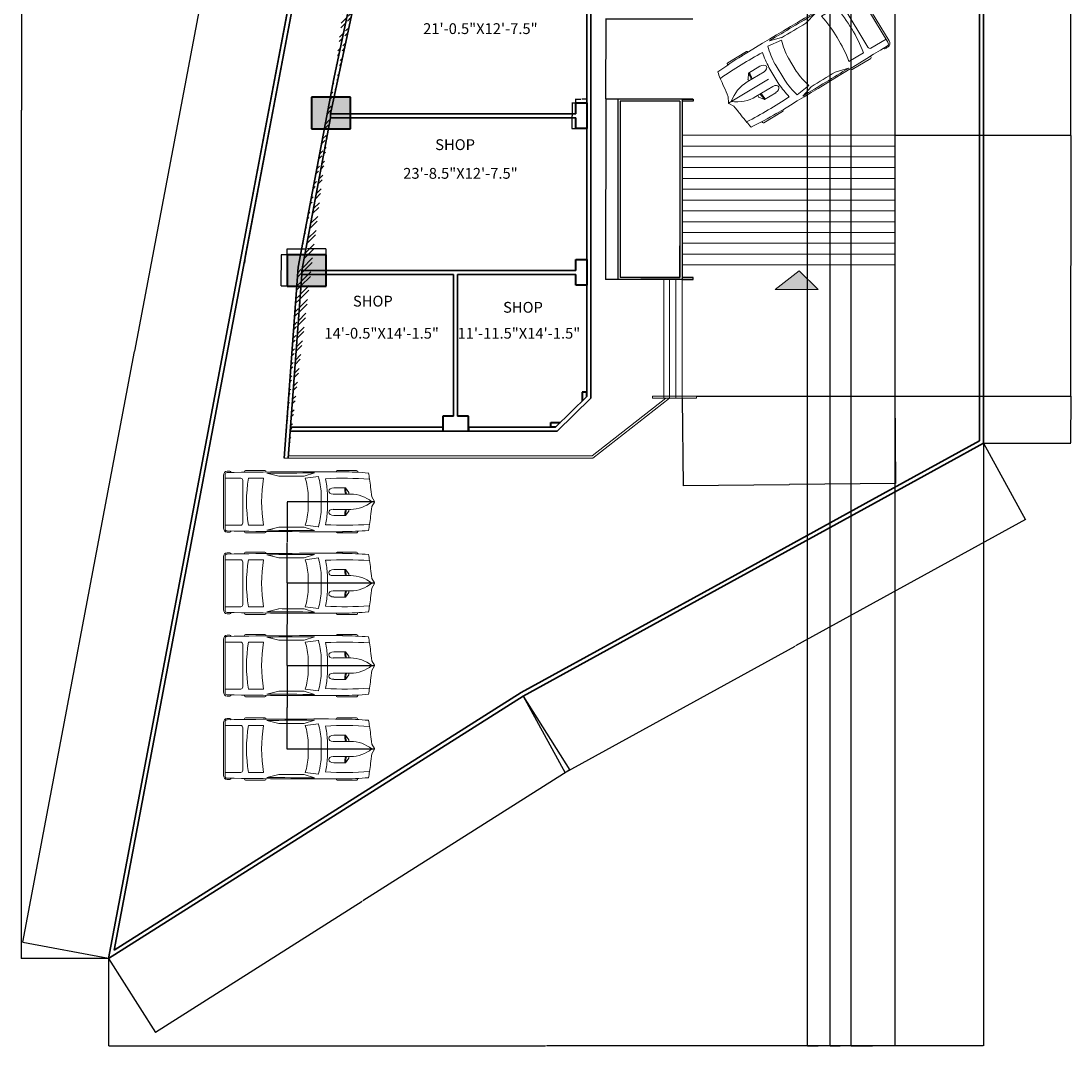
# Model space of a CAD drawing. Units: inches. Extents: x 1563 to 5866, y -225 to 2207.
# Tile 1 of 3: x 2993 to 4159, y -225 to 913. Entities that reach past the tile are written whole.
import ezdxf

# ---------------------------------------------------------------- set-up
doc = ezdxf.new("R2010")
doc.units = ezdxf.units.IN
for name, color, linetype, lineweight in [('A-ANNO-DIMS', 2, 'Continuous', 18), ('A-ANNO-SYMB', 7, 'Continuous', 18), ('A-AREA-IDEN', 7, 'Continuous', 18), ('A-COLS', 1, 'Continuous', 40), ('A-FLOR-STRS', 3, 'Continuous', 18), ('A-WALL', 7, 'Continuous', 35), ('A-WALL-INTR', 7, 'Continuous', 30), ('A-WALL-PATT', 8, 'Continuous', 13), ('C-PKNG', 8, 'Continuous', 25), ('C-PKNG-VEHI', 9, 'Continuous', 13), ('C-PROP', 2, 'Continuous', 35), ('C-SITE-PVMT', 9, 'Continuous', 18)]:
    doc.layers.add(name, color=color, linetype=linetype, lineweight=lineweight)
doc.styles.get("Standard").update_dxf_attribs({"font": 'arial.ttf'})
doc.dimstyles.get("Standard").update_dxf_attribs({"dimtxt": 0.18, "dimasz": 0.18, "dimexe": 0.18, "dimexo": 0.0625, "dimgap": 0.09, "dimtad": 0, "dimtih": 1, "dimtoh": 1, "dimdec": 4, "dimzin": 0, "dimdsep": 46, "dimtxsty": 'Standard', "dimcen": 0.09, "dimadec": 0, "dimazin": 0, "dimtfac": 1, "dimtdec": 4, "dimtofl": 0, "dimtmove": 0, "dimatfit": 3, "dimfxl": 1, "dimtolj": 1, "dimtzin": 0, "dimarcsym": 0})

# ---------------------------------------------------------------- blocks, each defined once
blk = doc.blocks.new('*U2')
for p, q in [((21.1, 37.4), (21.1, 36.8)), ((46.6, 38.9), (22.4, 38.9)), ((47.8, 37.4), (47.8, 37.4)), ((88, 31.9), (74.8, 35.9)), ((134.3, 35.6), (119.3, 31.8)), ((135.5, 37.1), (135.5, 37.4)), ((136.7, 38.9), (160.9, 38.9)), ((162.1, 37.4), (162.1, 36.8)), ((70, 31.5), (86.4, 29.4)), ((138.4, 29.4), (157.2, 29.4)), ((164.5, 26.4), (164.5, -26.4)), ((186.5, 29.4), (167, 29.4)), ((186.5, -33.5), (186.5, 33.5)), ((188.4, -32.8), (188.4, 32.8)), ((32.3, 11.6), (36.1, 17.2)), ((36.1, 17.2), (50.9, 17.2)), ((3.3, 6.1), (0.1, 0.4)), ((29.8, 9.5), (51.7, 9.5)), ((32.1, 9.5), (32.1, 11.2)), ((58.9, -10.8), (58.9, 10.8)), ((66.6, -10.5), (66.6, 10.5)), ((82.7, 8.5), (82.7, -8.5)), ((186.5, -10.5), (186.5, 10.5)), ((0, 0), (51.7, 0)), ((0.1, -0.4), (3.3, -6.1)), ((29.8, -9.5), (51.7, -9.5)), ((32.1, -9.5), (32.1, -11.2)), ((32.3, -11.6), (36.1, -17.2)), ((36.1, -17.2), (50.9, -17.2)), ((86.4, -29.4), (70, -31.5)), ((88, -31.9), (74.8, -35.9)), ((134.3, -35.6), (119.3, -31.8)), ((157.2, -29.4), (138.4, -29.4)), ((167, -29.4), (186.5, -29.4)), ((21.1, -37.4), (21.1, -36.8)), ((46.6, -38.9), (22.4, -38.9)), ((47.8, -37.4), (47.8, -37.4)), ((135.5, -37.1), (135.5, -37.4)), ((136.7, -38.9), (160.9, -38.9)), ((162.1, -37.4), (162.1, -36.8))]:
    blk.add_line(p, q)
for centre, major_axis, ratio, start_param, end_param in [((266, -27.5), (0, 313.3), 0.842304, 1.367076, 1.39176), ((41.2, -490.9), (0, 528.2), 0.842304, 0.00281, 0.075598), ((22.4, 37.4), (0, -1.48), 0.842304, 3.141593, 4.712389), ((64.5, -10555.6), (0, 10593), 0.842304, -0.013397, 0.002797), ((46.6, 37.4), (0, 1.48), 0.842304, -1.570796, 0), ((64.5, -10555.6), (0, -10591.5), 0.842304, 3.133765, 3.140441), ((136.7, 37.4), (0, -1.48), 0.842304, 3.141593, 4.712389), ((160.9, 37.4), (0, 1.48), 0.842304, -1.570796, 0), ((180.6, 35.8), (0, 2.22), 0.842304, -0.013017, 1.249894), ((64.5, -10556.4), (0, 10595.3), 0.842304, -0.013397, -0.013017), ((184, 32.8), (0, -5.25), 0.842304, 1.570796, 3.128196), ((184, 33.5), (0, -2.96), 0.842304, 1.570796, 3.128196), ((259.2, -27.5), (0, -305.3), 0.842304, 4.528606, 4.561838), ((37.5, -594), (0, -623.3), 0.842304, 3.096046, 3.200911), ((134.4, 5.4), (0, -89.8), 0.842304, 4.449482, 4.652344), ((135.3, 5.4), (0, 81.8), 0.842304, 1.245306, 1.50788), ((149.6, 2.8), (0, -79.6), 0.842304, 4.372215, 4.640744), ((95.8, -3666.4), (0, -3698.2), 0.842304, 3.134049, 3.144098), ((17.1, 0), (0, 147), 0.842304, 4.511394, 4.913384), ((35.9, 0), (0, 147), 0.842304, 4.511394, 4.913384), ((167, 26.4), (0, 2.96), 0.842304, 0, 1.570796), ((-204.5, 52.4), (0, -251), 0.842304, 1.385369, 1.434372), ((13, 17), (0, 27.4), 0.842304, 4.435146, 4.718221), ((14.2, 17), (0, 27.4), 0.842304, 4.435146, 4.718221), ((50.8, 13.3), (6.34, -0.36), 0.603834, -1.395552, 1.581315), ((0.6, 0), (0, -0.74), 0.842304, 4.131459, 5.293319), ((29.8, -46.7), (0, 56.2), 0.842304, 0, 0.590319), ((32.7, 11.2), (0, 0.74), 0.842304, 0.879714, 1.570796), ((-204.5, -52.4), (0, 251), 0.842304, -1.434372, -1.385369), ((29.8, 46.7), (0, 56.2), 0.842304, 2.551274, 3.141593), ((32.7, -11.2), (0, -0.74), 0.842304, 4.712389, 5.403472), ((13, -17), (0, -27.4), 0.842304, 1.564964, 1.848039), ((14.2, -17), (0, -27.4), 0.842304, 1.564964, 1.848039), ((134.4, -5.4), (0, -89.8), 0.842304, -1.510751, -1.307889), ((135.3, -5.4), (0, -81.8), 0.842304, -1.50788, -1.245306), ((149.6, -2.8), (0, -79.6), 0.842304, -1.499151, -1.230623), ((259.2, 27.5), (0, 305.3), 0.842304, 1.721348, 1.754579), ((266, 27.5), (0, 313.3), 0.842304, 1.749832, 1.774517), ((37.5, 594), (0, -623.3), 0.842304, -0.059319, 0.045547), ((95.8, 3666.4), (0, -3698.2), 0.842304, -0.002505, 0.007544), ((167, -26.4), (0, -2.96), 0.842304, 4.712389, 6.283185), ((184, -32.8), (0, -5.25), 0.842304, 0.013397, 1.570796), ((184, -33.5), (0, 2.96), 0.842304, 3.15499, 4.712389), ((41.2, 490.9), (0, -528.2), 0.842304, -0.075598, -0.00281), ((22.4, -37.4), (0, 1.48), 0.842304, 1.570796, 3.141593), ((64.5, 10555.6), (0, 10593), 0.842304, 3.138796, 3.15499), ((46.6, -37.4), (0, -1.48), 0.842304, 0, 1.570796), ((64.5, 10555.6), (0, -10591.5), 0.842304, 0.001152, 0.007828), ((136.7, -37.4), (0, -1.48), 0.842304, -1.570796, 0), ((160.9, -37.4), (0, 1.48), 0.842304, 3.141593, 4.712389), ((180.6, -35.8), (0, -2.22), 0.842304, -1.249894, 0.013017), ((64.5, 10556.4), (0, 10595.3), 0.842304, 3.15461, 3.15499)]:
    blk.add_ellipse(centre, major_axis=major_axis, ratio=ratio, start_param=start_param, end_param=end_param)
at = {"extrusion": (0, 0, -1)}
blk.add_ellipse((50.8, -13.3), major_axis=(6.34, 0.36), ratio=0.603834, start_param=-1.395552, end_param=1.581315, dxfattribs=at)
blk = doc.blocks.new('COL-RECT-FILLED')
h = blk.add_hatch(color=256)
h.dxf.hatch_style = 1
h.paths.add_polyline_path([(0, 34.9), (0, 0), (43.4, 0), (43.4, 34.9)])
for p, q in [((43.4, 34.9), (0, 34.9)), ((0, 34.9), (0, 0)), ((43.4, 0), (43.4, 34.9)), ((0, 0), (43.4, 0))]:
    blk.add_line(p, q)
blk = doc.blocks.new('PIER-SHOP-RETURN-2')
for p, q in [((0, 16.5), (0, 28.5)), ((0, 28.5), (12, 28.5)), ((12, 28.5), (12, 12)), ((0, 0), (0, 12)), ((12, 12), (12, 0)), ((12, 0), (0, 0))]:
    blk.add_line(p, q)
blk = doc.blocks.new('*D10')
at = {"layer": 'A-ANNO-DIMS', "color": 0, "lineweight": -2, "transparency": 16777216}
for p, q in [((3288.6, 653.6), (3288.6, 660.2)), ((3288.8, 660), (3309.2, 660)), ((3331.8, 660), (3311.4, 660)), ((3332, 653.6), (3332, 660.2))]:
    blk.add_line(p, q, dxfattribs=at)
at = {"layer": 'A-ANNO-DIMS', "color": 0, "transparency": 16777216}
for points in [[(3288.8, 660.1), (3288.8, 660), (3288.6, 660)], [(3331.8, 660.1), (3331.8, 660), (3332, 660)]]:
    blk.add_solid(points, dxfattribs=at)
at = {"layer": 'Defpoints', "color": 0, "transparency": 16777216}
for p in [(3288.6, 653.5), (3332, 660), (3332, 653.5)]:
    blk.add_point(p, dxfattribs=at)
at = {"layer": 'A-ANNO-DIMS', "color": 0, "transparency": 16777216, "insert": (3310.3, 660), "char_height": 0.18, "attachment_point": 5}
blk.add_mtext('\\A1;COLUMN 43 TYP.', dxfattribs=at)
blk = doc.blocks.new('*D11')
at = {"layer": 'A-ANNO-DIMS', "color": 0, "lineweight": -2, "transparency": 16777216}
for p, q in [((3288.6, 653.5), (3281.9, 653.5)), ((3282.1, 653.4), (3282.1, 636.3)), ((3282.1, 618.8), (3282.1, 635.9)), ((3288.6, 618.6), (3281.9, 618.6))]:
    blk.add_line(p, q, dxfattribs=at)
at = {"layer": 'A-ANNO-DIMS', "color": 0, "transparency": 16777216}
for points in [[(3282.1, 653.4), (3282.2, 653.4), (3282.1, 653.5)], [(3282.1, 618.8), (3282.2, 618.8), (3282.1, 618.6)]]:
    blk.add_solid(points, dxfattribs=at)
at = {"layer": 'Defpoints', "color": 0, "transparency": 16777216}
for p in [(3282.1, 653.5), (3288.6, 653.5), (3288.6, 618.6)]:
    blk.add_point(p, dxfattribs=at)
at = {"layer": 'A-ANNO-DIMS', "color": 0, "transparency": 16777216, "insert": (3282.1, 636.1), "char_height": 0.18, "attachment_point": 5}
blk.add_mtext('\\A1;35 TYP.', dxfattribs=at)
blk = doc.blocks.new('*D14')
at = {"layer": 'A-ANNO-DIMS', "color": 0, "lineweight": -2, "transparency": 16777216}
for p, q in [((3609.4, 822), (3605, 822)), ((3605.2, 821.8), (3605.2, 807.9)), ((3605.2, 793.7), (3605.2, 807.6)), ((3609.4, 793.5), (3605, 793.5))]:
    blk.add_line(p, q, dxfattribs=at)
at = {"layer": 'A-ANNO-DIMS', "color": 0, "transparency": 16777216}
for points in [[(3605.2, 821.8), (3605.2, 821.8), (3605.2, 822)], [(3605.2, 793.7), (3605.2, 793.7), (3605.2, 793.5)]]:
    blk.add_solid(points, dxfattribs=at)
at = {"layer": 'Defpoints', "color": 0, "transparency": 16777216}
for p in [(3605.2, 822), (3609.5, 822), (3609.5, 793.5)]:
    blk.add_point(p, dxfattribs=at)
at = {"layer": 'A-ANNO-DIMS', "color": 0, "transparency": 16777216, "insert": (3605.2, 807.8), "char_height": 0.18, "attachment_point": 5}
blk.add_mtext('\\A1;RETURN PIER 2 29 TYP.', dxfattribs=at)
blk = doc.blocks.new('*D15')
at = {"layer": 'A-ANNO-DIMS', "color": 0, "lineweight": -2, "transparency": 16777216}
for p, q in [((3609.5, 822.1), (3609.5, 826.5)), ((3609.7, 826.3), (3615, 826.3)), ((3621.3, 826.3), (3616, 826.3)), ((3621.5, 822.1), (3621.5, 826.5))]:
    blk.add_line(p, q, dxfattribs=at)
at = {"layer": 'A-ANNO-DIMS', "color": 0, "transparency": 16777216}
for points in [[(3609.7, 826.3), (3609.7, 826.3), (3609.5, 826.3)], [(3621.3, 826.3), (3621.3, 826.3), (3621.5, 826.3)]]:
    blk.add_solid(points, dxfattribs=at)
at = {"layer": 'Defpoints', "color": 0, "transparency": 16777216}
for p in [(3609.5, 822), (3621.5, 826.3), (3621.5, 822)]:
    blk.add_point(p, dxfattribs=at)
at = {"layer": 'A-ANNO-DIMS', "color": 0, "transparency": 16777216, "insert": (3615.5, 826.3), "char_height": 0.18, "attachment_point": 5}
blk.add_mtext('\\A1;12 TYP.', dxfattribs=at)
blk = doc.blocks.new('*D18')
at = {"layer": 'A-ANNO-DIMS', "color": 0, "lineweight": -2, "transparency": 16777216}
for p, q in [((4062.1, 444.2), (4062.1, -225.3)), ((3090.4, -128.3), (3090.4, -225.3)), ((3090.6, -225.1), (3575.8, -225.1)), ((4061.9, -225.1), (3576.6, -225.1))]:
    blk.add_line(p, q, dxfattribs=at)
at = {"layer": 'A-ANNO-DIMS', "color": 0, "transparency": 16777216}
for points in [[(3090.6, -225.1), (3090.6, -225.2), (3090.4, -225.1)], [(4061.9, -225.1), (4061.9, -225.2), (4062.1, -225.1)]]:
    blk.add_solid(points, dxfattribs=at)
at = {"layer": 'Defpoints', "color": 0, "transparency": 16777216}
for p in [(4062.1, 444.3), (3090.4, -128.2), (4062.1, -225.1)]:
    blk.add_point(p, dxfattribs=at)
at = {"layer": 'A-ANNO-DIMS', "color": 0, "transparency": 16777216, "insert": (3576.2, -225.1), "char_height": 0.18, "attachment_point": 5}
blk.add_mtext('\\A1;971.7', dxfattribs=at)
blk = doc.blocks.new('*D19')
at = {"layer": 'A-ANNO-DIMS', "color": 0, "lineweight": -2, "transparency": 16777216}
for p, q in [((3379.5, 1756.3), (2993.3, 1756.3)), ((2993.5, 1756.1), (2993.5, 814.2)), ((2993.5, -128), (2993.5, 813.9)), ((3090.3, -128.2), (2993.3, -128.2))]:
    blk.add_line(p, q, dxfattribs=at)
at = {"layer": 'A-ANNO-DIMS', "color": 0, "transparency": 16777216}
for points in [[(2993.4, 1756.1), (2993.5, 1756.1), (2993.5, 1756.3)], [(2993.4, -128), (2993.5, -128), (2993.5, -128.2)]]:
    blk.add_solid(points, dxfattribs=at)
at = {"layer": 'Defpoints', "color": 0, "transparency": 16777216}
for p in [(2993.5, 1756.3), (3379.6, 1756.3), (3090.4, -128.2)]:
    blk.add_point(p, dxfattribs=at)
at = {"layer": 'A-ANNO-DIMS', "color": 0, "transparency": 16777216, "insert": (2993.5, 814), "char_height": 0.18, "attachment_point": 5}
blk.add_mtext('\\A1;1884.5', dxfattribs=at)
blk = doc.blocks.new('*D23')
at = {"layer": 'A-ANNO-DIMS', "color": 0, "lineweight": -2, "transparency": 16777216}
for p, q in [((3727.5, 494), (3728.5, 397)), ((3963.5, 496.5), (3964.5, 399.5)), ((3728.7, 397.1), (3846.2, 398.4)), ((3964.3, 399.6), (3846.8, 398.4))]:
    blk.add_line(p, q, dxfattribs=at)
at = {"layer": 'A-ANNO-DIMS', "color": 0, "transparency": 16777216}
for points in [[(3728.7, 397.2), (3728.7, 397.1), (3728.5, 397.1)], [(3964.3, 399.7), (3964.3, 399.6), (3964.5, 399.6)]]:
    blk.add_solid(points, dxfattribs=at)
at = {"layer": 'Defpoints', "color": 0, "transparency": 16777216}
for p in [(3727.5, 494), (3963.5, 496.5), (3728.5, 397.1)]:
    blk.add_point(p, dxfattribs=at)
at = {"layer": 'A-ANNO-DIMS', "color": 0, "transparency": 16777216, "insert": (3846.5, 398.4), "char_height": 0.18, "attachment_point": 5}
blk.add_mtext('\\A1;236', dxfattribs=at)
blk = doc.blocks.new('*D27')
at = {"layer": 'A-ANNO-DIMS', "color": 0, "lineweight": -2, "transparency": 16777216}
for p, q in [((3963.5, 1691.8), (4159.1, 1691.8)), ((4159, 1691.6), (4159, 1239.2)), ((4159, 786.4), (4159, 1238.8)), ((3963.5, 786.2), (4159.1, 786.2))]:
    blk.add_line(p, q, dxfattribs=at)
at = {"layer": 'A-ANNO-DIMS', "color": 0, "transparency": 16777216}
for points in [[(4158.9, 1691.6), (4159, 1691.6), (4159, 1691.8)], [(4158.9, 786.4), (4159, 786.4), (4159, 786.2)]]:
    blk.add_solid(points, dxfattribs=at)
at = {"layer": 'Defpoints', "color": 0, "transparency": 16777216}
for p in [(3963.5, 1691.8), (4159, 1691.8), (3963.5, 786.2)]:
    blk.add_point(p, dxfattribs=at)
at = {"layer": 'A-ANNO-DIMS', "color": 0, "transparency": 16777216, "insert": (4159, 1239), "char_height": 0.18, "attachment_point": 5}
blk.add_mtext('\\A1;905.6', dxfattribs=at)
blk = doc.blocks.new('*D28')
at = {"layer": 'A-ANNO-DIMS', "color": 0, "lineweight": -2, "transparency": 16777216}
for p, q in [((3963.5, 786.2), (4159.1, 786.2)), ((4159, 786), (4159, 641.6)), ((4159, 496.7), (4159, 641.2)), ((3963.5, 496.5), (4159.1, 496.5))]:
    blk.add_line(p, q, dxfattribs=at)
at = {"layer": 'A-ANNO-DIMS', "color": 0, "transparency": 16777216}
for points in [[(4158.9, 786), (4159, 786), (4159, 786.2)], [(4158.9, 496.7), (4159, 496.7), (4159, 496.5)]]:
    blk.add_solid(points, dxfattribs=at)
at = {"layer": 'Defpoints', "color": 0, "transparency": 16777216}
for p in [(3963.5, 786.2), (4159, 786.2), (3963.5, 496.5)]:
    blk.add_point(p, dxfattribs=at)
at = {"layer": 'A-ANNO-DIMS', "color": 0, "transparency": 16777216, "insert": (4159, 641.4), "char_height": 0.18, "attachment_point": 5}
blk.add_mtext('\\A1;289.7', dxfattribs=at)
blk = doc.blocks.new('*D29')
at = {"layer": 'A-ANNO-DIMS', "color": 0, "lineweight": -2, "transparency": 16777216}
for p, q in [((3963.5, 496.5), (4159.1, 496.5)), ((4159, 496.4), (4159, 470.6)), ((4159, 444.5), (4159, 470.2)), ((4062.1, 444.3), (4159.1, 444.3))]:
    blk.add_line(p, q, dxfattribs=at)
at = {"layer": 'A-ANNO-DIMS', "color": 0, "transparency": 16777216}
for points in [[(4158.9, 496.4), (4159, 496.4), (4159, 496.5)], [(4158.9, 444.5), (4159, 444.5), (4159, 444.3)]]:
    blk.add_solid(points, dxfattribs=at)
at = {"layer": 'Defpoints', "color": 0, "transparency": 16777216}
for p in [(3963.5, 496.5), (4159, 496.5), (4062.1, 444.3)]:
    blk.add_point(p, dxfattribs=at)
at = {"layer": 'A-ANNO-DIMS', "color": 0, "transparency": 16777216, "insert": (4159, 470.4), "char_height": 0.18, "attachment_point": 5}
blk.add_mtext('\\A1;52.26', dxfattribs=at)
blk = doc.blocks.new('*D30')
at = {"layer": 'A-ANNO-DIMS', "color": 0, "lineweight": -2, "transparency": 16777216}
for p, q in [((3385.7, 197), (3288.7, 197.1)), ((3288.9, 196.9), (3288.8, 150.8)), ((3288.8, 104.5), (3288.8, 150.5)), ((3385.6, 104.2), (3288.6, 104.3))]:
    blk.add_line(p, q, dxfattribs=at)
at = {"layer": 'A-ANNO-DIMS', "color": 0, "transparency": 16777216}
for points in [[(3288.8, 196.9), (3288.9, 196.9), (3288.9, 197.1)], [(3288.8, 104.5), (3288.8, 104.5), (3288.8, 104.3)]]:
    blk.add_solid(points, dxfattribs=at)
at = {"layer": 'Defpoints', "color": 0, "transparency": 16777216}
for p in [(3288.9, 197.1), (3385.8, 197), (3385.7, 104.2)]:
    blk.add_point(p, dxfattribs=at)
at = {"layer": 'A-ANNO-DIMS', "color": 0, "transparency": 16777216, "insert": (3288.8, 150.7), "char_height": 0.18, "attachment_point": 5}
blk.add_mtext('\\A1;92.79', dxfattribs=at)
blk = doc.blocks.new('*D31')
at = {"layer": 'A-ANNO-DIMS', "color": 0, "lineweight": -2, "transparency": 16777216}
for p, q in [((3385.7, 288.8), (3288.7, 288.8)), ((3288.9, 288.6), (3288.9, 243.1)), ((3288.9, 197.2), (3288.9, 242.7)), ((3385.7, 197), (3288.7, 197))]:
    blk.add_line(p, q, dxfattribs=at)
at = {"layer": 'A-ANNO-DIMS', "color": 0, "transparency": 16777216}
for points in [[(3288.8, 288.6), (3288.9, 288.6), (3288.9, 288.8)], [(3288.8, 197.2), (3288.9, 197.2), (3288.9, 197)]]:
    blk.add_solid(points, dxfattribs=at)
at = {"layer": 'Defpoints', "color": 0, "transparency": 16777216}
for p in [(3288.9, 288.8), (3385.8, 288.8), (3385.8, 197)]:
    blk.add_point(p, dxfattribs=at)
at = {"layer": 'A-ANNO-DIMS', "color": 0, "transparency": 16777216, "insert": (3288.9, 242.9), "char_height": 0.18, "attachment_point": 5}
blk.add_mtext('\\A1;91.83', dxfattribs=at)
blk = doc.blocks.new('*D32')
at = {"layer": 'A-ANNO-DIMS', "color": 0, "lineweight": -2, "transparency": 16777216}
for p, q in [((3385.7, 379), (3288.7, 379)), ((3288.9, 378.8), (3288.9, 334.1)), ((3288.9, 289), (3288.9, 333.7)), ((3385.7, 288.8), (3288.7, 288.8))]:
    blk.add_line(p, q, dxfattribs=at)
at = {"layer": 'A-ANNO-DIMS', "color": 0, "transparency": 16777216}
for points in [[(3288.8, 378.8), (3288.9, 378.8), (3288.9, 379)], [(3288.8, 289), (3288.9, 289), (3288.9, 288.8)]]:
    blk.add_solid(points, dxfattribs=at)
at = {"layer": 'Defpoints', "color": 0, "transparency": 16777216}
for p in [(3288.9, 379), (3385.8, 379), (3385.8, 288.8)]:
    blk.add_point(p, dxfattribs=at)
at = {"layer": 'A-ANNO-DIMS', "color": 0, "transparency": 16777216, "insert": (3288.9, 333.9), "char_height": 0.18, "attachment_point": 5}
blk.add_mtext('\\A1;90.17', dxfattribs=at)
blk = doc.blocks.new('*D33')
at = {"layer": 'A-ANNO-DIMS', "color": 0, "lineweight": -2, "transparency": 16777216}
for p, q in [((3550.8, 163.2), (3602.7, 81.2)), ((3602.5, 81.3), (3372.7, -64.2)), ((3142.4, -210), (3372.1, -64.6)), ((3090.4, -128.3), (3142.3, -210.3))]:
    blk.add_line(p, q, dxfattribs=at)
at = {"layer": 'A-ANNO-DIMS', "color": 0, "transparency": 16777216}
for points in [[(3602.4, 81.3), (3602.5, 81.2), (3602.6, 81.4)], [(3142.3, -210), (3142.4, -210), (3142.2, -210.1)]]:
    blk.add_solid(points, dxfattribs=at)
at = {"layer": 'Defpoints', "color": 0, "transparency": 16777216}
for p in [(3550.8, 163.2), (3090.4, -128.2), (3142.2, -210.1)]:
    blk.add_point(p, dxfattribs=at)
at = {"layer": 'A-ANNO-DIMS', "color": 0, "transparency": 16777216, "insert": (3372.4, -64.4), "char_height": 0.18, "attachment_point": 5}
blk.add_mtext('\\A1;544.9', dxfattribs=at)
blk = doc.blocks.new('*D34')
at = {"layer": 'A-ANNO-DIMS', "color": 0, "lineweight": -2, "transparency": 16777216}
for p, q in [((4062.1, 444.2), (4108.8, 359.2)), ((4108.6, 359.3), (3853.4, 219)), ((3597.6, 78.4), (3852.8, 218.7)), ((3550.8, 163.2), (3597.5, 78.2))]:
    blk.add_line(p, q, dxfattribs=at)
at = {"layer": 'A-ANNO-DIMS', "color": 0, "transparency": 16777216}
for points in [[(4108.6, 359.3), (4108.6, 359.2), (4108.7, 359.4)], [(3597.6, 78.4), (3597.6, 78.4), (3597.5, 78.3)]]:
    blk.add_solid(points, dxfattribs=at)
at = {"layer": 'Defpoints', "color": 0, "transparency": 16777216}
for p in [(4062.1, 444.3), (3550.8, 163.2), (3597.5, 78.3)]:
    blk.add_point(p, dxfattribs=at)
at = {"layer": 'A-ANNO-DIMS', "color": 0, "transparency": 16777216, "insert": (3853.1, 218.8), "char_height": 0.18, "attachment_point": 5}
blk.add_mtext('\\A1;583.4', dxfattribs=at)
blk = doc.blocks.new('*D35')
at = {"layer": 'A-ANNO-DIMS', "color": 0, "lineweight": -2, "transparency": 16777216}
for p, q in [((3243.1, 1202.5), (3119.2, 546.4)), ((3338.3, 1184.7), (3243, 1202.7)), ((2995.2, -110.1), (3119.1, 546)), ((3090.3, -128.2), (2995, -110.2))]:
    blk.add_line(p, q, dxfattribs=at)
at = {"layer": 'A-ANNO-DIMS', "color": 0, "transparency": 16777216}
for points in [[(3243.1, 1202.5), (3243.2, 1202.5), (3243.2, 1202.7)], [(2995.2, -110.1), (2995.2, -110.1), (2995.2, -110.2)]]:
    blk.add_solid(points, dxfattribs=at)
at = {"layer": 'Defpoints', "color": 0, "transparency": 16777216}
for p in [(3243.2, 1202.7), (3338.4, 1184.7), (3090.4, -128.2)]:
    blk.add_point(p, dxfattribs=at)
at = {"layer": 'A-ANNO-DIMS', "color": 0, "transparency": 16777216, "insert": (3119.2, 546.2), "char_height": 0.18, "attachment_point": 5}
blk.add_mtext('\\A1;1336', dxfattribs=at)
blk = doc.blocks.new('*D42')
at = {"layer": 'A-ANNO-DIMS', "color": 0, "lineweight": -2, "transparency": 16777216}
for p, q in [((3739.4, 915), (3642.4, 915)), ((3642.6, 914.8), (3642.6, 870.8)), ((3642.6, 826.6), (3642.6, 870.5)), ((3739.4, 826.4), (3642.4, 826.4))]:
    blk.add_line(p, q, dxfattribs=at)
at = {"layer": 'A-ANNO-DIMS', "color": 0, "transparency": 16777216}
for points in [[(3642.5, 914.8), (3642.6, 914.8), (3642.6, 915)], [(3642.5, 826.6), (3642.6, 826.6), (3642.6, 826.4)]]:
    blk.add_solid(points, dxfattribs=at)
at = {"layer": 'Defpoints', "color": 0, "transparency": 16777216}
for p in [(3642.6, 915), (3739.5, 915), (3739.5, 826.4)]:
    blk.add_point(p, dxfattribs=at)
at = {"layer": 'A-ANNO-DIMS', "color": 0, "transparency": 16777216, "insert": (3642.6, 870.7), "char_height": 0.18, "attachment_point": 5}
blk.add_mtext('\\A1;88.58', dxfattribs=at)
blk = doc.blocks.new('*D43')
at = {"layer": 'A-ANNO-DIMS', "color": 0, "lineweight": -2, "transparency": 16777216}
for p, q in [((3739.4, 826.4), (3642.4, 826.4)), ((3642.6, 826.2), (3642.6, 726.3)), ((3642.6, 626.1), (3642.6, 725.9)), ((3739.4, 625.9), (3642.4, 625.9))]:
    blk.add_line(p, q, dxfattribs=at)
at = {"layer": 'A-ANNO-DIMS', "color": 0, "transparency": 16777216}
for points in [[(3642.5, 826.2), (3642.6, 826.2), (3642.6, 826.4)], [(3642.5, 626.1), (3642.6, 626.1), (3642.6, 625.9)]]:
    blk.add_solid(points, dxfattribs=at)
at = {"layer": 'Defpoints', "color": 0, "transparency": 16777216}
for p in [(3642.6, 826.4), (3739.5, 826.4), (3739.5, 625.9)]:
    blk.add_point(p, dxfattribs=at)
at = {"layer": 'A-ANNO-DIMS', "color": 0, "transparency": 16777216, "insert": (3642.6, 726.1), "char_height": 0.18, "attachment_point": 5}
blk.add_mtext('\\A1;200.5', dxfattribs=at)
blk = doc.blocks.new('*D45')
at = {"layer": 'A-ANNO-DIMS', "color": 0, "lineweight": -2, "transparency": 16777216}
for p, q in [((3891.5, 1506.9), (3891.5, -225.3)), ((3914.9, 1506.9), (3914.9, -225.3)), ((3891.7, -225.1), (3902.8, -225.1)), ((3914.8, -225.1), (3903.6, -225.1))]:
    blk.add_line(p, q, dxfattribs=at)
at = {"layer": 'A-ANNO-DIMS', "color": 0, "transparency": 16777216}
for points in [[(3891.7, -225.1), (3891.7, -225.2), (3891.5, -225.1)], [(3914.8, -225.1), (3914.8, -225.2), (3914.9, -225.1)]]:
    blk.add_solid(points, dxfattribs=at)
at = {"layer": 'Defpoints', "color": 0, "transparency": 16777216}
for p in [(3891.5, 1507), (3914.9, 1507), (3914.9, -225.1)]:
    blk.add_point(p, dxfattribs=at)
at = {"layer": 'A-ANNO-DIMS', "color": 0, "transparency": 16777216, "insert": (3903.2, -225.1), "char_height": 0.18, "attachment_point": 5}
blk.add_mtext('\\A1;23.42', dxfattribs=at)
blk = doc.blocks.new('*D47')
at = {"layer": 'A-ANNO-DIMS', "color": 0, "lineweight": -2, "transparency": 16777216}
for p, q in [((3866.4, 1506.9), (3866.4, -225.3)), ((3891.5, 1506.9), (3891.5, -225.3)), ((3866.6, -225.1), (3878.5, -225.1)), ((3891.4, -225.1), (3879.4, -225.1))]:
    blk.add_line(p, q, dxfattribs=at)
at = {"layer": 'A-ANNO-DIMS', "color": 0, "transparency": 16777216}
for points in [[(3866.6, -225.1), (3866.6, -225.2), (3866.4, -225.1)], [(3891.4, -225.1), (3891.4, -225.2), (3891.5, -225.1)]]:
    blk.add_solid(points, dxfattribs=at)
at = {"layer": 'Defpoints', "color": 0, "transparency": 16777216}
for p in [(3866.4, 1507), (3891.5, 1507), (3891.5, -225.1)]:
    blk.add_point(p, dxfattribs=at)
at = {"layer": 'A-ANNO-DIMS', "color": 0, "transparency": 16777216, "insert": (3879, -225.1), "char_height": 0.18, "attachment_point": 5}
blk.add_mtext('\\A1;25.113', dxfattribs=at)
blk = doc.blocks.new('*D48')
at = {"layer": 'A-ANNO-DIMS', "color": 0, "lineweight": -2, "transparency": 16777216}
for p, q in [((3914.9, 1506.9), (3914.9, -225.3)), ((3963.5, 1506.9), (3963.5, -225.3)), ((3915.1, -225.1), (3938.8, -225.1)), ((3963.3, -225.1), (3939.6, -225.1))]:
    blk.add_line(p, q, dxfattribs=at)
at = {"layer": 'A-ANNO-DIMS', "color": 0, "transparency": 16777216}
for points in [[(3915.1, -225.1), (3915.1, -225.2), (3914.9, -225.1)], [(3963.3, -225.1), (3963.3, -225.2), (3963.5, -225.1)]]:
    blk.add_solid(points, dxfattribs=at)
at = {"layer": 'Defpoints', "color": 0, "transparency": 16777216}
for p in [(3914.9, 1507), (3963.5, 1507), (3963.5, -225.1)]:
    blk.add_point(p, dxfattribs=at)
at = {"layer": 'A-ANNO-DIMS', "color": 0, "transparency": 16777216, "insert": (3939.2, -225.1), "char_height": 0.18, "attachment_point": 5}
blk.add_mtext('\\A1;48.53', dxfattribs=at)

msp = doc.modelspace()

# ---------------------------------------------------------------- hatches: boundary and pattern name
at = {"layer": 'A-ANNO-SYMB'}
h = msp.add_hatch(color=256, dxfattribs=at)
h.dxf.hatch_style = 1
h.paths.add_polyline_path([(3857.3464, 635.5038), (3830.7817, 614.7966), (3878.6358, 614.7966)])
at = {"layer": 'A-WALL-PATT'}
h = msp.add_hatch(dxfattribs=at)
h.set_pattern_fill('ANSI32', color=256)
edge = h.paths.add_edge_path()
edge.add_line((3443.9794, 1691.8133), (3431.9794, 1530.0177))
edge.add_line((3439.4917, 1692.1461), (3423.9855, 1483.0764))
edge.add_line((3431.9794, 1525.5177), (3424.4794, 1434.0177))
edge.add_line((3423.9855, 1483.0764), (3420.4644, 1440.1194))
edge.add_line((3420.4644, 1440.1194), (3412.6295, 1270.5497))
edge.add_line((3424.4794, 1429.5177), (3417.4794, 1278.0177))
edge.add_line((3417.4794, 1273.5177), (3400.9794, 1122.0177))
edge.add_line((3412.6295, 1270.5497), (3395.5183, 1113.4377))
edge.add_line((3400.9794, 1117.5177), (3368.9794, 966.0177))
edge.add_line((3395.5183, 1113.4377), (3364.5765, 966.9477))
edge.add_line((3368.9794, 966.0177), (3368.9794, 961.5177))
edge.add_line((3364.5765, 966.9477), (3364.5765, 962.4477))
edge.add_line((3368.9794, 961.5177), (3336.9794, 810.0177))
edge.add_line((3364.5765, 962.4477), (3340.6094, 848.9784))
edge.add_line((3340.6094, 848.9784), (3301.0547, 639.5806))
edge.add_line((3336.9794, 810.0177), (3336.9794, 805.5177))
edge.add_line((3336.9794, 805.5177), (3304.9794, 636.1136))
edge.add_line((3301.0547, 639.5806), (3285.4229, 427.6136))
edge.add_line((3304.9794, 636.1136), (3304.9794, 631.6136))
edge.add_line((3304.9794, 631.6136), (3289.9351, 427.6136))

# ---------------------------------------------------------------- linework, layer by layer
at = {"layer": 'A-ANNO-SYMB'}
for p, q in [((3857.3464, 635.5038), (3830.7817, 614.7966)), ((3878.6358, 614.7966), (3857.3464, 635.5038)), ((3830.7817, 614.7966), (3878.6358, 614.7966))]:
    msp.add_line(p, q, dxfattribs=at)
at = {"layer": 'A-COLS'}
for p, q in [((3621.4794, 500.9392), (3616.4794, 500.9392)), ((3616.4794, 500.9392), (3616.4794, 491.0803)), ((3621.4794, 495.9392), (3621.4794, 500.9392)), ((3473.4794, 474.1136), (3461.4794, 474.1136)), ((3461.4794, 474.1136), (3461.4794, 457.6136)), ((3489.9794, 474.1136), (3477.9794, 474.1136)), ((3489.9794, 462.1136), (3489.9794, 474.1136)), ((3581.6718, 462.1136), (3581.6718, 467.1136)), ((3581.6718, 467.1136), (3591.8169, 467.1136)), ((3489.9794, 462.1136), (3489.9794, 457.6136)), ((3489.9794, 457.6136), (3489.9794, 462.1136)), ((3586.6718, 462.1136), (3581.6718, 462.1136))]:
    msp.add_line(p, q, dxfattribs=at)
at = {"layer": 'A-FLOR-STRS'}
for p, q in [((3727.4794, 786.2146), (3963.4794, 786.2146)), ((3727.4794, 774.2146), (3963.4794, 774.2146)), ((3727.4794, 762.2146), (3963.4794, 762.2146)), ((3727.4794, 750.2146), (3963.4794, 750.2146)), ((3727.4794, 738.2146), (3963.4794, 738.2146)), ((3727.4794, 726.2146), (3963.4794, 726.2146)), ((3727.4794, 714.2146), (3963.4794, 714.2146)), ((3727.4794, 702.2146), (3963.4794, 702.2146)), ((3727.4794, 690.2146), (3963.4794, 690.2146)), ((3727.4794, 678.2146), (3963.4794, 678.2146)), ((3727.4794, 666.2146), (3963.4794, 666.2146)), ((3727.4794, 654.2146), (3963.4794, 654.2146)), ((3727.4794, 642.2146), (3963.4794, 642.2146))]:
    msp.add_line(p, q, dxfattribs=at)
at = {"layer": 'A-WALL'}
for p, q in [((3621.4794, 1687.3133), (3621.4794, 495.9392)), ((3625.9794, 1687.3133), (3625.9794, 494.0374)), ((3368.9794, 961.5177), (3336.9794, 810.0177)), ((3364.5765, 962.4477), (3340.6094, 848.9784)), ((3340.6094, 848.9784), (3301.0547, 639.5806)), ((3336.9794, 805.5177), (3304.9794, 636.1136)), ((3336.9794, 810.0177), (3336.9794, 805.5177)), ((3301.0547, 639.5806), (3285.4229, 427.6136)), ((3304.9794, 631.6136), (3289.9351, 427.6136)), ((3304.9794, 636.1136), (3304.9794, 631.6136)), ((3621.4794, 495.9392), (3586.6718, 462.1136)), ((3625.9794, 494.0374), (3588.4981, 457.6136)), ((3292.4794, 457.6136), (3292.1475, 457.6136)), ((3461.4794, 462.1136), (3292.4794, 462.1136)), ((3292.4794, 457.6136), (3588.4981, 457.6136)), ((3586.6718, 462.1136), (3489.9794, 462.1136))]:
    msp.add_line(p, q, dxfattribs=at)
at = {"layer": 'A-WALL-INTR'}
for p, q in [((3609.4794, 810.0177), (3336.9794, 810.0177)), ((3336.9794, 810.0177), (3336.9794, 805.5177)), ((3336.9794, 805.5177), (3609.4794, 805.5177)), ((3473.4794, 636.1136), (3304.9794, 636.1136)), ((3304.9794, 636.1136), (3304.9794, 631.6136)), ((3304.9794, 631.6136), (3473.4794, 631.6136)), ((3609.4794, 636.1136), (3473.4794, 636.1136)), ((3473.4794, 631.6136), (3473.4794, 474.1136)), ((3477.9794, 631.6136), (3609.4794, 631.6136)), ((3477.9794, 631.6136), (3477.9794, 474.1136))]:
    msp.add_line(p, q, dxfattribs=at)
at = {"layer": 'C-PKNG'}
for p, q in [((3963.4794, 1691.8133), (3963.4794, 496.5374)), ((3727.4794, 826.3734), (3655.9794, 826.3734)), ((3655.9794, 826.3734), (3655.9794, 625.8734)), ((3724.9794, 823.8734), (3658.4794, 823.8734)), ((3658.4794, 823.8734), (3658.4794, 628.3734)), ((3724.9794, 823.8734), (3724.9794, 628.3734)), ((3727.4794, 826.3734), (3727.4794, 625.8734)), ((3727.4794, 826.3734), (3739.4794, 826.3734)), ((3739.4794, 823.8734), (3727.4794, 823.8734)), ((3739.4794, 826.3734), (3739.4794, 823.8734)), ((3724.7155, 628.3734), (3724.7155, 663.306)), ((3727.4794, 625.8734), (3655.9794, 625.8734)), ((3724.9794, 628.3734), (3658.4794, 628.3734)), ((3681.3396, 628.3734), (3724.7155, 628.3734)), ((3739.4794, 628.3734), (3727.4794, 628.3734)), ((3727.4794, 625.8734), (3739.4794, 625.8734)), ((3739.4794, 625.8734), (3739.4794, 628.3734)), ((3743.4809, 496.5374), (3963.4794, 496.5374))]:
    msp.add_line(p, q, dxfattribs=at)
at = {"layer": 'C-PROP'}
for p, q in [((4057.5619, 446.938), (4057.5619, 1751.8133)), ((4062.0619, 444.2765), (4062.0619, 1756.3133)), ((3338.4478, 1185.0285), (3237.6755, 651.5527)), ((3342.8696, 1184.1932), (3242.0973, 650.7174)), ((3330.967, 1121.1824), (3096.721, -118.8872)), ((3242.0973, 650.7174), (3241.2172, 643.9933))]:
    msp.add_line(p, q, dxfattribs=at)
for points in [[(3326.5452, 1122.0177), (3090.3766, -128.2295), (3550.7842, 163.2371), (3788.3855, 293.8419), (3941.0013, 377.7319), (4062.0619, 444.2765)], [(3096.721, -118.8872), (3548.4947, 167.1136), (3786.2178, 297.7854), (3938.8336, 381.6754), (4057.5619, 446.938)]]:
    msp.add_lwpolyline(points, dxfattribs=at)
at = {"layer": 'C-SITE-PVMT'}
for p, q in [((3707.1784, 625.8734), (3707.1784, 494.0374)), ((3713.4207, 625.8734), (3713.4207, 494.0374)), ((3720.3377, 625.8734), (3720.3377, 494.0374)), ((3727.4794, 625.8734), (3727.4794, 494.0374)), ((3709.3544, 494.0374), (3627.3557, 430.1136)), ((3713.4207, 494.0374), (3628.215, 427.6136)), ((3694.4525, 496.5374), (3743.4809, 496.5374)), ((3694.4525, 496.5374), (3694.4525, 494.0374)), ((3694.4525, 494.0374), (3743.4809, 494.0374)), ((3743.4809, 496.5374), (3743.4809, 494.0374)), ((3292.4794, 427.6136), (3285.4229, 427.6136)), ((3290.1195, 430.1136), (3588.4981, 430.1136)), ((3292.4794, 427.6136), (3588.4981, 427.6136)), ((3588.4981, 430.1136), (3627.3557, 430.1136)), ((3588.4981, 427.6136), (3628.215, 427.6136))]:
    msp.add_line(p, q, dxfattribs=at)

# ---------------------------------------------------------------- block references
at = {"layer": 'A-COLS'}
for name, p in [('COL-RECT-FILLED', (3315.7909, 793.4935)), ('PIER-SHOP-RETURN-2', (3609.4794, 793.5177)), ('COL-RECT-FILLED', (3288.6291, 618.6026)), ('PIER-SHOP-RETURN-2', (3609.4794, 619.6136))]:
    msp.add_blockref(name, p, dxfattribs=at)
at = {"layer": 'C-PKNG-VEHI', "rotation": 31.07575251048744}
msp.add_blockref('*U2', (3778.9297, 821.878), dxfattribs=at)
at = {"layer": 'C-PKNG-VEHI', "xscale": -0.8904152165417734, "yscale": 0.8904152165417734, "zscale": 0.8904152165417734}
for p in [(3385.795, 379.1745), (3385.795, 288.6333), (3385.795, 197.1757), (3385.795, 104.5754)]:
    msp.add_blockref('*U2', p, dxfattribs=at)

# ---------------------------------------------------------------- texts
at = {"layer": 'A-AREA-IDEN'}
for s, p in [('21\'-0.5"X12\'-7.5"', (3439.717, 898.5972)), ('SHOP', (3453.1377, 769.7452)), ('23\'-8.5"X12\'-7.5"', (3417.586, 737.8782)), ('SHOP', (3361.7725, 595.9376)), ('SHOP', (3528.5486, 589.0894)), ('14\'-0.5"X14\'-1.5"', (3330.0835, 560.3023)), ('11\'-11.5"X14\'-1.5"', (3477.9794, 560.3023))]:
    msp.add_text(s, height=12, dxfattribs=at).set_placement(p)

# ---------------------------------------------------------------- dimensions: what is measured, and where the dimension line sits
at = {"layer": 'A-ANNO-DIMS'}
for base, p1, p2, angle, override, picture, middle in [((2993.4766, 1756.3133), (3090.3766, -128.2295), (3379.5737, 1756.3133), 90, {"dimdec": 1, "dimlfac": 1, "dimrnd": 0, "dimzin": 0, "dimdsep": 46, "dimlunit": 2}, '*D19', (2993.4766, 814.0419)), ((4158.9619, 1691.8133), (3963.4794, 786.2146), (3963.4794, 1691.8133), 90, {"dimdec": 1, "dimlfac": 1, "dimrnd": 0, "dimzin": 0, "dimdsep": 46, "dimlunit": 2}, '*D27', (4158.9619, 1239.0139)), ((3243.1801, 1202.6675), (3090.3766, -128.2295), (3338.396, 1184.6804), 79.3024241, {"dimdec": 0, "dimlfac": 1, "dimrnd": 0, "dimzin": 0, "dimdsep": 46, "dimlunit": 2}, '*D35', (3119.1704, 546.2125)), ((3642.5794, 914.9515), (3739.4794, 826.3734), (3739.4794, 914.9515), 90, {"dimdec": 2, "dimlfac": 1, "dimrnd": 0, "dimzin": 0, "dimdsep": 46, "dimlunit": 2}, '*D42', (3642.5794, 870.6624)), ((3642.5794, 826.3734), (3739.4794, 625.8734), (3739.4794, 826.3734), 90, {"dimdec": 1, "dimlfac": 1, "dimrnd": 0, "dimzin": 0, "dimdsep": 46, "dimlunit": 2}, '*D43', (3642.5794, 726.1234)), ((4158.9619, 786.2146), (3963.4794, 496.5374), (3963.4794, 786.2146), 90, {"dimdec": 1, "dimlfac": 1, "dimrnd": 0, "dimzin": 0, "dimdsep": 46, "dimlunit": 2}, '*D28', (4158.9619, 641.376)), ((3728.5058, 397.1428), (3963.4794, 496.5374), (3727.4794, 494.0374), 180.6069241, {"dimdec": 0, "dimlfac": 1, "dimrnd": 0, "dimzin": 0, "dimdsep": 46, "dimlunit": 2}, '*D23', (3846.5058, 398.3928)), ((4158.9619, 496.5374), (4062.0619, 444.2765), (3963.4794, 496.5374), 90, {"dimdec": 2, "dimlfac": 1, "dimrnd": 0, "dimzin": 0, "dimdsep": 46, "dimlunit": 2}, '*D29', (4158.9619, 470.407)), ((3597.4613, 78.3203), (4062.0619, 444.2765), (3550.7842, 163.2371), 208.7967421, {"dimdec": 1, "dimlfac": 1, "dimrnd": 0, "dimzin": 0, "dimdsep": 46, "dimlunit": 2}, '*D34', (3853.1002, 218.8401)), ((3288.8722, 378.9877), (3385.7722, 288.8201), (3385.7722, 378.9877), 90, {"dimdec": 2, "dimlfac": 1, "dimrnd": 0, "dimzin": 0, "dimdsep": 46, "dimlunit": 2}, '*D32', (3288.8722, 333.9039)), ((3288.8722, 288.8201), (3385.7722, 196.9888), (3385.7722, 288.8201), 90, {"dimdec": 2, "dimlfac": 1, "dimrnd": 0, "dimzin": 0, "dimdsep": 46, "dimlunit": 2}, '*D31', (3288.8722, 242.9045)), ((3288.8723, 197.0601), (3385.704, 104.2012), (3385.7722, 196.9888), 89.957839, {"dimdec": 2, "dimlfac": 1, "dimrnd": 0, "dimzin": 0, "dimdsep": 46, "dimlunit": 2}, '*D30', (3288.8381, 150.6663)), ((3142.2073, -210.1025), (3550.7842, 163.2371), (3090.3766, -128.2295), 212.336355, {"dimdec": 1, "dimlfac": 1, "dimrnd": 0, "dimzin": 0, "dimdsep": 46, "dimlunit": 2}, '*D33', (3372.4111, -64.3692))]:
    dim = msp.add_linear_dim(base=base, p1=p1, p2=p2, angle=angle, dimstyle='Standard', override=override, dxfattribs=at)
    dim.commit()
    dim.dimension.update_dxf_attribs({"geometry": picture, "text_midpoint": middle})
for base, p1, p2, override, picture, middle in [((3891.5309, -225.1295), (3866.4183, 1506.9516), (3891.5309, 1506.9516), {"dimdec": 3, "dimlfac": 1, "dimrnd": 0, "dimzin": 0, "dimdsep": 46, "dimlunit": 2}, '*D47', (3878.9746, -225.1295)), ((3914.9489, -225.1295), (3891.5309, 1506.9516), (3914.9489, 1506.9516), {"dimdec": 2, "dimlfac": 1, "dimrnd": 0, "dimzin": 0, "dimdsep": 46, "dimlunit": 2}, '*D45', (3903.2399, -225.1295)), ((3963.4794, -225.1295), (3914.9489, 1506.9516), (3963.4794, 1506.9516), {"dimdec": 2, "dimlfac": 1, "dimrnd": 0, "dimzin": 0, "dimdsep": 46, "dimlunit": 2}, '*D48', (3939.2141, -225.1295)), ((4062.0619, -225.1295), (3090.3766, -128.2295), (4062.0619, 444.2765), {"dimdec": 1, "dimlfac": 1, "dimrnd": 0, "dimzin": 0, "dimdsep": 46, "dimlunit": 2}, '*D18', (3576.2193, -225.1295))]:
    dim = msp.add_linear_dim(base=base, p1=p1, p2=p2, dimstyle='Standard', override=override, dxfattribs=at)
    dim.commit()
    dim.dimension.update_dxf_attribs({"geometry": picture, "text_midpoint": middle})
for base, p1, p2, text, picture, middle in [((3605.2043818998, 822.0176943851), (3609.4793818998, 793.5176943851), (3609.4793818998, 822.0176943851), 'RETURN PIER 2 <> TYP.', '*D14', (3605.2043818998, 807.7676943851)), ((3282.1227, 653.5353), (3288.6291, 618.6026), (3288.6291, 653.5353), '<> TYP.', '*D11', (3282.1227, 636.069))]:
    dim = msp.add_linear_dim(base=base, p1=p1, p2=p2, angle=90, text=text, dimstyle='Standard', override={"dimdec": 0, "dimlfac": 1, "dimrnd": 0, "dimzin": 0, "dimdsep": 46, "dimlunit": 2}, dxfattribs=at)
    dim.commit()
    dim.dimension.update_dxf_attribs({"geometry": picture, "text_midpoint": middle})
for base, p1, p2, text, picture, middle in [((3621.4794, 826.2927), (3609.4794, 822.0177), (3621.4794, 822.0177), '<> TYP.', '*D15', (3615.4794, 826.2927)), ((3332.005, 660.0417), (3288.6291, 653.5353), (3332.005, 653.5353), 'COLUMN <> TYP.', '*D10', (3310.3171, 660.0417))]:
    dim = msp.add_linear_dim(base=base, p1=p1, p2=p2, text=text, dimstyle='Standard', override={"dimdec": 0, "dimlfac": 1, "dimrnd": 0, "dimzin": 0, "dimdsep": 46, "dimlunit": 2}, dxfattribs=at)
    dim.commit()
    dim.dimension.update_dxf_attribs({"geometry": picture, "text_midpoint": middle})

doc.saveas('drawing.dxf')
